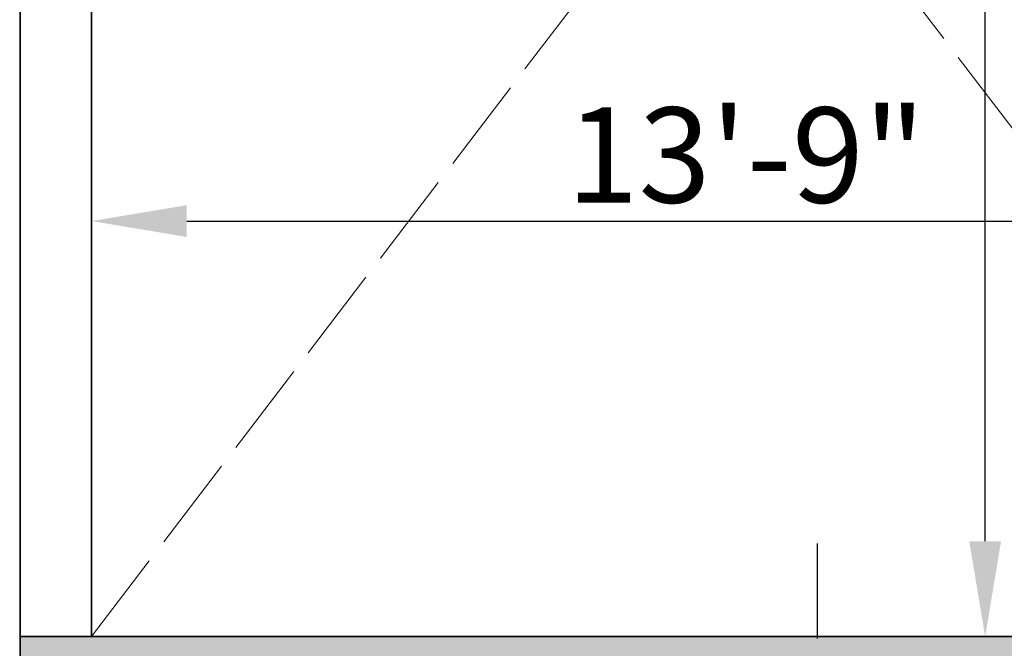
# Model space of a CAD drawing. Units: inches. Extents: x 2083 to 3317, y 1141 to 2115.
# Tile 248 of 256: x 2944 to 3068, y 1485 to 1564. Entities that reach past the tile are written whole.
import ezdxf

# ---------------------------------------------------------------- set-up
doc = ezdxf.new("R2010")
doc.units = ezdxf.units.IN
doc.linetypes.add('ACAD_ISO02W100', pattern=[15, 12, -3])
for name, color, linetype, lineweight in [('A-ANNO-DIMS', 2, 'Continuous', 18), ('A-FLOR-OPEN', 8, 'ACAD_ISO02W100', 13), ('A-WALL', 7, 'Continuous', 35)]:
    doc.layers.add(name, color=color, linetype=linetype, lineweight=lineweight)
doc.layers.add('A-WALL-PATT', color=251, linetype='Continuous', lineweight=13, true_color=0x636466)
doc.styles.get("Standard").update_dxf_attribs({"font": 'arial.ttf'})
doc.dimstyles.new('ISO-25', dxfattribs={"dimtxt": 12, "dimasz": 12, "dimexe": 1.25, "dimexo": 0.625, "dimtad": 1, "dimlunit": 3, "dimtxsty": 'Standard', "dimcen": 2.5, "dimadec": 0, "dimazin": 0, "dimtfac": 1, "dimtmove": 0, "dimatfit": 3, "dimfxl": 1, "dimarcsym": 0})

# ---------------------------------------------------------------- blocks, each defined once
blk = doc.blocks.new('*D18')
at = {"layer": 'A-ANNO-DIMS', "color": 0, "lineweight": -2, "transparency": 16777216}
for p, q in [((3018.48, 1456.16), (3018.48, 1452.14)), ((3041.07, 1456.16), (3041.07, 1452.14)), ((3006.48, 1453.39), (2828.36, 1453.39)), ((3041.07, 1453.39), (3018.48, 1453.39)), ((3053.07, 1453.39), (3065.07, 1453.39))]:
    blk.add_line(p, q, dxfattribs=at)
at = {"layer": 'A-ANNO-DIMS', "color": 0, "transparency": 16777216}
for points in [[(3006.48, 1455.39), (3006.48, 1451.39), (3018.48, 1453.39)], [(3053.07, 1455.39), (3053.07, 1451.39), (3041.07, 1453.39)]]:
    blk.add_solid(points, dxfattribs=at)
at = {"layer": 'Defpoints', "color": 0, "transparency": 16777216}
for p in [(3018.48, 1456.78), (3041.07, 1456.78), (3018.48, 1453.39)]:
    blk.add_point(p, dxfattribs=at)
at = {"layer": 'A-ANNO-DIMS', "color": 0, "transparency": 16777216, "insert": (2911.42, 1460.22), "char_height": 12, "attachment_point": 5}
blk.add_mtext('BASIN 1\'-10 1/2" TYP.', dxfattribs=at)
blk = doc.blocks.new('*D19')
at = {"layer": 'A-ANNO-DIMS', "color": 0, "lineweight": -2, "transparency": 16777216}
for p, q in [((3044.46, 1486.5), (3044.46, 1498.5)), ((3041.69, 1474.5), (3045.71, 1474.5)), ((3044.46, 1474.5), (3044.46, 1456.78)), ((3041.69, 1456.78), (3045.71, 1456.78)), ((3044.46, 1444.78), (3044.46, 1331.55))]:
    blk.add_line(p, q, dxfattribs=at)
at = {"layer": 'A-ANNO-DIMS', "color": 0, "transparency": 16777216}
for points in [[(3042.46, 1486.5), (3046.46, 1486.5), (3044.46, 1474.5)], [(3042.46, 1444.78), (3046.46, 1444.78), (3044.46, 1456.78)]]:
    blk.add_solid(points, dxfattribs=at)
at = {"layer": 'Defpoints', "color": 0, "transparency": 16777216}
for p in [(3041.07, 1474.5), (3041.07, 1456.78), (3044.46, 1456.78)]:
    blk.add_point(p, dxfattribs=at)
at = {"layer": 'A-ANNO-DIMS', "color": 0, "transparency": 16777216, "insert": (3037.63, 1382.17), "char_height": 12, "attachment_point": 5, "rotation": 90}
blk.add_mtext('1\'-5 1/2" TYP.', dxfattribs=at)
blk = doc.blocks.new('*D46')
at = {"layer": 'A-ANNO-DIMS', "color": 0, "lineweight": -2, "transparency": 16777216}
for p, q in [((2952.96, 1487.39), (2952.96, 1540.36)), ((3117.96, 1487.39), (3117.96, 1540.36)), ((2964.96, 1539.11), (3105.96, 1539.11))]:
    blk.add_line(p, q, dxfattribs=at)
at = {"layer": 'A-ANNO-DIMS', "color": 0, "transparency": 16777216}
for points in [[(2964.96, 1541.11), (2964.96, 1537.11), (2952.96, 1539.11)], [(3105.96, 1541.11), (3105.96, 1537.11), (3117.96, 1539.11)]]:
    blk.add_solid(points, dxfattribs=at)
at = {"layer": 'Defpoints', "color": 0, "transparency": 16777216}
for p in [(3117.96, 1539.11), (2952.96, 1486.76), (3117.96, 1486.76)]:
    blk.add_point(p, dxfattribs=at)
at = {"layer": 'A-ANNO-DIMS', "color": 0, "transparency": 16777216, "insert": (3035.46, 1545.87), "char_height": 12, "attachment_point": 5}
blk.add_mtext('13\'-9"', dxfattribs=at)
blk = doc.blocks.new('*D65')
at = {"layer": 'A-ANNO-DIMS', "color": 0, "lineweight": -2, "transparency": 16777216}
for p, q in [((3117.33, 1702.76), (3064.36, 1702.76)), ((3065.61, 1498.76), (3065.61, 1690.76)), ((3117.33, 1486.76), (3064.36, 1486.76))]:
    blk.add_line(p, q, dxfattribs=at)
at = {"layer": 'A-ANNO-DIMS', "color": 0, "transparency": 16777216}
for points in [[(3063.61, 1690.76), (3067.61, 1690.76), (3065.61, 1702.76)], [(3063.61, 1498.76), (3067.61, 1498.76), (3065.61, 1486.76)]]:
    blk.add_solid(points, dxfattribs=at)
at = {"layer": 'Defpoints', "color": 0, "transparency": 16777216}
for p in [(3065.61, 1702.76), (3117.96, 1702.76), (3117.96, 1486.76)]:
    blk.add_point(p, dxfattribs=at)
at = {"layer": 'A-ANNO-DIMS', "color": 0, "transparency": 16777216, "insert": (3058.86, 1594.76), "char_height": 12, "attachment_point": 5, "rotation": 90}
blk.add_mtext('18\'-0"', dxfattribs=at)

msp = doc.modelspace()

# ---------------------------------------------------------------- hatches: boundary and pattern name
at = {"layer": 'A-WALL-PATT'}
h = msp.add_hatch(color=256, dxfattribs=at)
h.dxf.hatch_style = 1
h.paths.add_polyline_path([(3126.96, 2020.761), (2748.96, 2020.761), (2604.96, 2020.761), (2226.96, 2020.761), (2226.96, 1702.761), (2466.96, 1702.761), (2466.96, 1582.761), (2418.96, 1582.761), (2418.96, 1477.761), (2226.96, 1477.761), (2226.96, 1263.261), (2544.96, 1263.261), (2544.96, 1411.761), (2604.96, 1411.761), (2685.96, 1411.761), (2685.96, 1420.761), (2604.96, 1420.761), (2604.96, 1573.761), (2604.96, 1702.761), (2604.96, 2011.761), (2748.96, 2011.761), (2748.96, 1702.761), (2862.96, 1702.761), (2862.96, 1621.761), (2871.96, 1621.761), (2871.96, 1702.761), (2883.96, 1702.761), (2883.96, 1706.939, -0.0264593), (2883.96, 1711.761), (2757.96, 1711.761), (2757.96, 1807.761), (2787.96, 1807.761), (2787.96, 1812.261), (2757.96, 1812.261), (2757.96, 2011.761), (2877.96, 2011.761), (2877.96, 1812.261), (2847.96, 1812.261), (2847.96, 1807.761), (2889.836, 1807.761), (2889.836, 1812.261), (2882.46, 1812.261), (2882.46, 2011.761), (3117.96, 2011.761), (3117.96, 1812.261), (2937.836, 1812.261), (2937.836, 1807.761), (2995.71, 1807.761), (2995.71, 1796.118), (3000.21, 1796.118), (3000.21, 1807.761), (3117.96, 1807.761), (3117.96, 1711.761), (3000.21, 1711.761), (3000.21, 1760.118), (2998.573, 1760.118, -0.020711), (2995.71, 1760.118), (2995.71, 1711.761), (2931.96, 1711.761), (2931.96, 1702.761), (3126.96, 1702.761)])
h.paths.add_polyline_path([(2471.46, 2011.761), (2471.46, 1810.011), (2462.717, 1810.011), (2462.717, 1805.511), (2505.96, 1805.511), (2505.96, 1810.011), (2475.96, 1810.011), (2475.96, 2011.761), (2595.96, 2011.761), (2595.96, 1810.011), (2565.96, 1810.011), (2565.96, 1805.511), (2595.96, 1805.511), (2595.96, 1711.761), (2235.96, 1711.761), (2235.96, 1805.511), (2353.71, 1805.511), (2353.71, 1796.054), (2358.21, 1796.054), (2358.21, 1805.511), (2414.717, 1805.511), (2414.717, 1810.011), (2235.96, 1810.011), (2235.96, 2011.761)], flags=16)
h.paths.add_polyline_path([(2270.205, 1994.61), (2270.205, 1970.61), (2246.205, 1970.61), (2246.205, 1994.61)], flags=0)
edge = h.paths.add_edge_path(flags=0)
edge.add_ellipse((2332.027, 1899.798), major_axis=(-3.043, 3.043), ratio=0.1682525, start_angle=-161.33217, end_angle=-156.30711, ccw=False)
edge.add_ellipse((2333.082, 1898.744), major_axis=(-1.055, 1.055), ratio=0.4535321, start_angle=-123.37102, end_angle=-94.15911)
edge = h.paths.add_edge_path(flags=0)
edge.add_ellipse((2332.027, 1968.876), major_axis=(3.043, 3.043), ratio=0.1682525, start_angle=18.66783, end_angle=23.69289)
edge.add_spline(control_points=[(2332.926, 1970.691), (2332.227, 1970.336), (2330.894, 1969.659), (2328.413, 1970.932), (2327.204, 1967.749), (2324.71, 1969.956), (2322.533, 1967.012), (2320.013, 1971.296), (2317.68, 1968.158), (2316.041, 1967.102), (2315.427, 1966.81)], knot_values=[0, 0, 0, 0, 2.2670587, 4.3245589, 6.6855835, 8.8786411, 11.121502, 14.300359, 17.7552837, 19.732645, 19.732645, 19.732645, 19.732645], degree=3, periodic=0)
edge.add_ellipse((2332.027, 1968.876), major_axis=(3.043, 3.043), ratio=0.1682525, start_angle=18.66783, end_angle=23.69289, ccw=False)
edge.add_ellipse((2333.082, 1969.931), major_axis=(1.055, 1.055), ratio=0.4535321, start_angle=56.62898, end_angle=85.84089, ccw=False)
edge = h.paths.add_edge_path(flags=0)
edge.add_spline(control_points=[(2296.428, 1967.988), (2293.628, 1965.336), (2287.704, 1959.727), (2299.744, 1949.996), (2294.533, 1935.669), (2290.573, 1920.604), (2293.394, 1909.974), (2296.185, 1904.967)], knot_values=[0.0991853, 0.0991853, 0.0991853, 0.0991853, 0.3453009, 0.6198217, 0.9826526, 1.3860932, 1.8105546, 1.8105546, 1.8105546, 1.8105546], degree=3, periodic=0)
edge.add_spline(control_points=[(2296.185, 1904.967), (2297.384, 1902.619), (2298.001, 1901.949), (2298.553, 1901.468)], knot_values=[0.0062457, 0.0062457, 0.0062457, 0.0062457, 0.0554759, 0.0554759, 0.0554759, 0.0554759], degree=3, periodic=0)
edge.add_spline(control_points=[(2298.553, 1901.468), (2297.259, 1900.923), (2295.225, 1900.232), (2293.06, 1900.614), (2292.101, 1900.788), (2292.09, 1900.791)], knot_values=[0.3128349, 0.3128349, 0.3128349, 0.3128349, 0.4017797, 0.4749867, 0.4759027, 0.4759027, 0.4759027, 0.4759027], degree=3, periodic=0)
edge.add_arc((2292.794, 1904.664), 3.937, 215.4209, 259.69818, ccw=False)
edge.add_spline(control_points=[(2289.585, 1902.382), (2289.477, 1902.535), (2289.368, 1902.688), (2289.261, 1902.841)], knot_values=[0.1028719, 0.1028719, 0.1028719, 0.1028719, 0.1168958, 0.1168958, 0.1168958, 0.1168958], degree=3, periodic=0)
edge.add_spline(control_points=[(2289.261, 1902.841), (2288.687, 1902.55), (2287.64, 1902.02), (2285.881, 1901.874), (2283.853, 1901.504), (2281.72, 1899.711), (2278.467, 1899.493), (2276.157, 1901.883), (2272.259, 1899.804), (2267.778, 1901.843), (2262.244, 1900.184), (2257.415, 1901.782), (2254.318, 1900.726), (2253.178, 1900.337)], knot_values=[0, 0, 0, 0, 1.9079767, 3.4771759, 5.261074, 7.9728515, 11.6802485, 13.7179214, 16.9395917, 22.789562, 27.5025027, 33.5952153, 37.1456181, 37.1456181, 37.1456181, 37.1456181], degree=3, periodic=0)
edge.add_line((2253.178, 1900.337), (2250.244, 1902.841))
edge.add_line((2250.244, 1902.841), (2250.244, 1965.833))
edge.add_line((2250.244, 1965.833), (2253.178, 1968.337))
edge.add_spline(control_points=[(2253.178, 1968.337), (2254.318, 1967.948), (2257.415, 1966.892), (2262.244, 1968.49), (2267.778, 1966.831), (2271.527, 1968.537), (2273.876, 1967.828), (2274.207, 1967.728)], knot_values=[0, 0, 0, 0, 0.0901802, 0.2449351, 0.3646438, 0.5132331, 0.5378548, 0.5378548, 0.5378548, 0.5378548], degree=3, periodic=0)
edge.add_arc((2274.353, 1963.793), 3.937, 72.05113, 92.12795, ccw=False)
edge.add_arc((2281.297, 1985.23), 18.596, 252.05113, 288.56572)
edge.add_arc((2292.317, 1956.029), 12.646, 71.02679, 113.77822, ccw=False)
edge = h.paths.add_edge_path(flags=0)
edge.add_spline(control_points=[(2274.899, 1951.856), (2275.066, 1951.617), (2275.233, 1951.377), (2275.398, 1951.136)], knot_values=[1.4099157, 1.4099157, 1.4099157, 1.4099157, 1.4315903, 1.4315903, 1.4315903, 1.4315903], degree=3, periodic=0)
edge.add_spline(control_points=[(2275.398, 1951.136), (2275.792, 1950.562), (2276.179, 1949.984), (2276.546, 1949.397)], knot_values=[1.3582378, 1.3582378, 1.3582378, 1.3582378, 1.4099157, 1.4099157, 1.4099157, 1.4099157], degree=3, periodic=0)
edge.add_line((2276.546, 1949.397), (2277.437, 1947.862))
edge.add_spline(control_points=[(2277.437, 1947.862), (2276.304, 1945.673), (2274.64, 1942.427), (2274.632, 1938.094), (2272.799, 1930.852), (2274.356, 1943.897), (2275.948, 1947.923), (2276.546, 1949.397)], knot_values=[0.0056315, 0.0056315, 0.0056315, 0.0056315, 0.1860139, 0.2660015, 0.3570872, 0.5963902, 0.7397317, 0.7397317, 0.7397317, 0.7397317], degree=3, periodic=0)
edge.add_spline(control_points=[(2276.546, 1949.397), (2276.179, 1949.984), (2275.792, 1950.562), (2275.398, 1951.136)], knot_values=[1.3582378, 1.3582378, 1.3582378, 1.3582378, 1.4099157, 1.4099157, 1.4099157, 1.4099157], degree=3, periodic=0)
edge.add_spline(control_points=[(2275.398, 1951.136), (2274.943, 1950.08), (2274.208, 1948.025), (2273.935, 1944.851), (2272.469, 1937.627), (2273.466, 1945.696), (2274.701, 1951.059), (2274.899, 1951.856)], knot_values=[0.1043639, 0.1043639, 0.1043639, 0.1043639, 0.1896363, 0.2696239, 0.3607096, 0.6000126, 0.6446217, 0.6446217, 0.6446217, 0.6446217], degree=3, periodic=0)
h.paths.add_polyline_path([(2269.168, 1963.128, -0.3575267), (2268.171, 1960.976, -0.0925607), (2268.171, 1939.436, -0.3575267), (2269.168, 1937.285, -0.3575267), (2267.016, 1938.282, -0.1647847), (2254.686, 1938.282, -0.3575267), (2252.534, 1937.285, -0.3575267), (2253.531, 1939.436, -0.0925607), (2253.531, 1960.976, -0.3575267), (2252.534, 1963.128, -0.3575267), (2254.686, 1962.131, -0.1647847), (2267.016, 1962.131, -0.3575267)], flags=0)
h.paths.add_polyline_path([(2248.874, 1967.802), (2248.874, 1957.028), (2249.458, 1957.028), (2249.458, 1911.647), (2248.874, 1911.647), (2248.874, 1900.873), (2246.512, 1900.873, 0.1973271), (2244.15, 1902.457), (2244.15, 1966.218, 0.1973271), (2246.512, 1967.802)], flags=0)
h.paths.add_polyline_path([(2269.168, 1931.389, -0.3575267), (2268.171, 1929.238, -0.0925607), (2268.171, 1907.698, -0.3575267), (2269.168, 1905.547, -0.3575267), (2267.016, 1906.544, -0.1647847), (2254.686, 1906.544, -0.3575267), (2252.534, 1905.547, -0.3575267), (2253.531, 1907.698, -0.0925607), (2253.531, 1929.238, -0.3575267), (2252.534, 1931.389, -0.3575267), (2254.686, 1930.392, -0.1647847), (2267.016, 1930.392, -0.3575267)], flags=0)
edge = h.paths.add_edge_path(flags=0)
edge.add_spline(control_points=[(2276.197, 1906.724), (2276.168, 1909.029), (2276.114, 1913.372), (2270.598, 1924.925), (2273.905, 1919.013), (2275.922, 1916.262), (2275.475, 1912.402), (2277.258, 1910.381), (2276.696, 1908.225), (2276.646, 1906.813), (2276.618, 1906.008)], knot_values=[0, 0, 0, 0, 8.6102597, 16.2212739, 18.8430575, 23.8048978, 27.4408283, 29.3561016, 31.2034776, 33.6506866, 33.6506866, 33.6506866, 33.6506866], degree=3, periodic=0)
edge.add_spline(control_points=[(2276.618, 1906.008), (2276.623, 1905.624), (2276.498, 1904.629), (2275.442, 1903.855), (2274.937, 1903.08), (2274.859, 1902.841)], knot_values=[0.1564884, 0.1564884, 0.1564884, 0.1564884, 0.1843975, 0.2313765, 0.2505985, 0.2505985, 0.2505985, 0.2505985], degree=3, periodic=0)
edge.add_line((2274.859, 1902.841), (2276.506, 1902.841))
edge.add_spline(control_points=[(2276.506, 1902.841), (2276.788, 1903.085), (2277.665, 1904.125), (2278.25, 1904.341), (2277.654, 1908.527), (2278.156, 1906.228), (2278.1, 1905.286), (2278.847, 1904.069), (2277.857, 1903.415), (2277.874, 1902.991), (2277.904, 1902.841)], knot_values=[0.0595743, 0.0595743, 0.0595743, 0.0595743, 0.0807529, 0.1037415, 0.1697201, 0.1760361, 0.2071372, 0.2404744, 0.2623409, 0.2736605, 0.2736605, 0.2736605, 0.2736605], degree=3, periodic=0)
edge.add_line((2277.904, 1902.841), (2280.03, 1902.841))
edge.add_spline(control_points=[(2280.03, 1902.841), (2279.888, 1903.088), (2279.499, 1903.982), (2280.152, 1905.939), (2278.104, 1909.658), (2279.762, 1907.185), (2280.328, 1904.875), (2280.485, 1903.49), (2281.463, 1903.249), (2281.758, 1902.936), (2281.834, 1902.841)], knot_values=[0.013856, 0.013856, 0.013856, 0.013856, 0.0348738, 0.0888667, 0.1078792, 0.1267378, 0.158714, 0.1937575, 0.2174868, 0.2267221, 0.2267221, 0.2267221, 0.2267221], degree=3, periodic=0)
edge.add_spline(control_points=[(2281.834, 1902.841), (2281.788, 1902.827), (2281.647, 1902.783), (2281.396, 1902.859), (2281.088, 1902.985), (2280.721, 1903.061), (2280.333, 1903.026), (2280.125, 1902.899), (2280.03, 1902.841)], knot_values=[0, 0, 0, 0, 0.1441304, 0.435517, 0.7492759, 1.1530457, 1.5483707, 1.878348, 1.878348, 1.878348, 1.878348], degree=3, periodic=0)
edge.add_line((2280.03, 1902.841), (2277.904, 1902.841))
edge.add_spline(control_points=[(2277.904, 1902.841), (2277.893, 1902.796), (2277.865, 1902.68), (2277.607, 1902.687), (2277.274, 1902.801), (2276.838, 1902.62), (2276.584, 1902.789), (2276.506, 1902.841)], knot_values=[0, 0, 0, 0, 0.1271885, 0.3261988, 0.6280094, 1.2435704, 1.5153306, 1.5153306, 1.5153306, 1.5153306], degree=3, periodic=0)
edge.add_line((2276.506, 1902.841), (2274.859, 1902.841))
edge.add_spline(control_points=[(2274.859, 1902.841), (2274.814, 1902.899), (2274.725, 1903.013), (2274.493, 1903.119), (2274.244, 1902.961), (2273.937, 1903.185), (2273.614, 1902.983), (2273.408, 1902.883), (2273.322, 1902.841)], knot_values=[0, 0, 0, 0, 0.2184302, 0.4369566, 0.6879766, 0.9903786, 1.3983955, 1.6918498, 1.6918498, 1.6918498, 1.6918498], degree=3, periodic=0)
edge.add_spline(control_points=[(2273.322, 1902.841), (2273.617, 1903.446), (2274.274, 1904.538), (2276.027, 1904.574), (2276.207, 1906.584), (2276.197, 1906.724)], knot_values=[0.0122268, 0.0122268, 0.0122268, 0.0122268, 0.0594721, 0.1062177, 0.134458, 0.134458, 0.134458, 0.134458], degree=3, periodic=0)
h.paths.add_polyline_path([(2270.776, 1897.79), (2270.776, 1873.79), (2246.776, 1873.79), (2246.776, 1897.79)], flags=0)
h.paths.add_polyline_path([(2353.71, 1760.005), (2353.71, 1760.054), (2358.21, 1760.054, -0.033729)], flags=0)
h.paths.add_polyline_path([(2321.819, 1737.529), (2341.995, 1737.529, -0.4142136), (2343.203, 1736.321), (2343.203, 1721.021, -0.4142136), (2341.995, 1719.813), (2321.819, 1719.813, -0.4142136), (2320.611, 1721.021), (2320.611, 1736.321, -0.4142136)], flags=0)
h.paths.add_polyline_path([(2324.235, 1736.321), (2339.579, 1736.321, -0.4142136), (2341.995, 1733.905), (2341.995, 1725.45, -0.4142136), (2339.579, 1723.034), (2333.681, 1723.034), (2333.845, 1722.045, -0.8706461), (2335.425, 1721.826, -0.767327), (2333.923, 1721.423), (2331.291, 1721.423, -0.767327), (2329.788, 1721.826, -0.8706461), (2331.368, 1722.045), (2331.533, 1723.034), (2324.235, 1723.034, -0.4142136), (2321.819, 1725.45), (2321.819, 1733.905, -0.4142136)], flags=0)
h.paths.add_polyline_path([(2570.484, 1928.615), (2589.684, 1928.615), (2590.169, 1928.615), (2590.169, 1904.993), (2570.484, 1904.993)], flags=0)
h.paths.add_polyline_path([(2574.447, 1927.264, -1), (2572.829, 1927.264, -1)], flags=0)
h.paths.add_polyline_path([(2573.09, 1926.941), (2573.925, 1927.776), (2574.148, 1927.553), (2573.313, 1926.718)], flags=0)
h.paths.add_polyline_path([(2578.779, 1919.73, -1), (2571.592, 1919.73, -1)], flags=0)
h.paths.add_polyline_path([(2578.385, 1919.73, -1), (2571.985, 1919.73, -1)], flags=0)
h.paths.add_polyline_path([(2331.596, 1729.476, -1), (2333.618, 1729.476, -1)], flags=0)
h.paths.add_polyline_path([(2578.034, 1927.264, -1), (2576.416, 1927.264, -1)], flags=0)
h.paths.add_polyline_path([(2576.689, 1927.531), (2576.912, 1927.754), (2577.747, 1926.919), (2577.524, 1926.696)], flags=0)
h.paths.add_polyline_path([(2578.139, 1909.86, -1), (2572.232, 1909.86, -1)], flags=0)
h.paths.add_polyline_path([(2577.745, 1909.86, -1), (2572.625, 1909.86, -1)], flags=0)
h.paths.add_polyline_path([(2583.798, 1927.264, -1), (2582.179, 1927.264, -1)], flags=0)
h.paths.add_polyline_path([(2582.719, 1927.754), (2583.554, 1926.919), (2583.331, 1926.696), (2582.496, 1927.531)], flags=0)
h.paths.add_polyline_path([(2582.496, 1927.531), (2582.719, 1927.754), (2583.554, 1926.919), (2583.331, 1926.696)], flags=0)
h.paths.add_polyline_path([(2587.739, 1920.53, -1), (2581.832, 1920.53, -1)], flags=0)
h.paths.add_polyline_path([(2587.345, 1920.53, -1), (2582.225, 1920.53, -1)], flags=0)
h.paths.add_polyline_path([(2587.385, 1927.264, -1), (2585.766, 1927.264, -1)], flags=0)
h.paths.add_polyline_path([(2586.082, 1926.98), (2586.917, 1927.815), (2587.14, 1927.593), (2586.305, 1926.758)], flags=0)
h.paths.add_polyline_path([(2588.379, 1910.66, -1), (2581.192, 1910.66, -1)], flags=0)
h.paths.add_polyline_path([(2587.985, 1910.66, -1), (2581.585, 1910.66, -1)], flags=0)
h.paths.add_polyline_path([(2417.168, 1729.478), (2437.344, 1729.478, -0.4142136), (2438.552, 1728.27), (2438.552, 1712.969, -0.4142136), (2437.344, 1711.761), (2417.168, 1711.761, -0.4142136), (2415.96, 1712.969), (2415.96, 1728.27, -0.4142136)], flags=0)
h.paths.add_polyline_path([(2419.584, 1728.27), (2434.928, 1728.27, -0.4142136), (2437.344, 1725.854), (2437.344, 1717.398, -0.4142136), (2434.928, 1714.983), (2429.029, 1714.983), (2429.194, 1713.994, -0.8706461), (2430.774, 1713.775, -0.767327), (2429.271, 1713.372), (2426.64, 1713.372, -0.767327), (2425.137, 1713.775, -0.8706461), (2426.717, 1713.994), (2426.882, 1714.983), (2419.584, 1714.983, -0.4142136), (2417.168, 1717.398), (2417.168, 1725.854, -0.4142136)], flags=0)
h.paths.add_polyline_path([(2419.584, 1728.27), (2434.928, 1728.27, -0.4142136), (2437.344, 1725.854), (2437.344, 1717.398, -0.4142136), (2434.928, 1714.983), (2429.029, 1714.983), (2428.358, 1719.009), (2427.553, 1719.009), (2426.882, 1714.983), (2419.584, 1714.983, -0.4142136), (2417.168, 1717.398), (2417.168, 1725.854, -0.4142136)], flags=0)
h.paths.add_polyline_path([(2426.944, 1721.425, -1), (2428.967, 1721.425, -1)], flags=0)
h.paths.add_polyline_path([(2475.96, 1702.761), (2595.96, 1702.761), (2595.96, 1582.761), (2475.96, 1582.761)], flags=16)
h.paths.add_polyline_path([(2427.96, 1573.761), (2595.96, 1573.761), (2595.96, 1468.761), (2595.96, 1420.761), (2384.46, 1420.761), (2384.46, 1468.761), (2427.96, 1468.761)], flags=16)
h.paths.add_polyline_path([(2379.96, 1468.761), (2379.96, 1420.761), (2235.96, 1420.761), (2235.96, 1468.761)], flags=16)
h.paths.add_polyline_path([(2317.816, 1466.696), (2337.992, 1466.696, -0.4142136), (2339.2, 1465.488), (2339.2, 1450.187, -0.4142136), (2337.992, 1448.979), (2317.816, 1448.979, -0.4142136), (2316.608, 1450.187), (2316.608, 1465.488, -0.4142136)], flags=0)
h.paths.add_polyline_path([(2320.232, 1465.488), (2335.576, 1465.488, -0.4142136), (2337.992, 1463.072), (2337.992, 1454.616, -0.4142136), (2335.576, 1452.2), (2329.677, 1452.2), (2329.842, 1451.212, -0.8706461), (2331.422, 1450.992, -0.767327), (2329.92, 1450.59), (2327.288, 1450.59, -0.767327), (2325.785, 1450.992, -0.8706461), (2327.365, 1451.212), (2327.53, 1452.2), (2320.232, 1452.2, -0.4142136), (2317.816, 1454.616), (2317.816, 1463.072, -0.4142136)], flags=0)
h.paths.add_polyline_path([(2320.232, 1465.488), (2335.576, 1465.488, -0.4142136), (2337.992, 1463.072), (2337.992, 1454.616, -0.4142136), (2335.576, 1452.2), (2329.677, 1452.2), (2329.006, 1456.227), (2328.201, 1456.227), (2327.53, 1452.2), (2320.232, 1452.2, -0.4142136), (2317.816, 1454.616), (2317.816, 1463.072, -0.4142136)], flags=0)
h.paths.add_polyline_path([(2327.593, 1458.643, -1), (2329.615, 1458.643, -1)], flags=0)
h.paths.add_polyline_path([(2244.412, 1433.34), (2241.921, 1433.34, -0.4142136), (2240.018, 1435.244), (2240.018, 1440.953, -0.4142105), (2241.921, 1442.856), (2244.412, 1442.856, -1.9764724)], flags=0)
h.paths.add_polyline_path([(2245.357, 1434.398, -0.4142136), (2245.357, 1441.799, -2.1440985)], flags=0)
h.paths.add_polyline_path([(2535.96, 1416.261), (2535.96, 1272.261), (2235.96, 1272.261), (2235.96, 1416.261)], flags=16)
h.paths.add_polyline_path([(2260.12, 1384.293), (2260.12, 1362.039), (2237.865, 1362.039), (2237.865, 1384.293)], flags=0)
edge = h.paths.add_edge_path(flags=0)
edge.add_line((2318.252, 1362.093), (2318.146, 1362.001))
edge.add_ellipse((2317.445, 1360.431), major_axis=(2.822, 2.822), ratio=0.1682525, start_angle=18.66783, end_angle=20.94813, ccw=False)
edge.add_ellipse((2318.423, 1361.409), major_axis=(0.978, 0.978), ratio=0.4535321, start_angle=56.62898, end_angle=70.2262, ccw=False)
edge = h.paths.add_edge_path(flags=0)
edge.add_line((2319.107, 1295.571), (2319.015, 1295.677))
edge.add_ellipse((2317.445, 1296.378), major_axis=(-2.822, 2.822), ratio=0.1682525, start_angle=-161.33217, end_angle=-159.05187, ccw=False)
edge.add_ellipse((2318.423, 1295.4), major_axis=(-0.978, 0.978), ratio=0.4535321, start_angle=-123.37102, end_angle=-109.7738)
edge = h.paths.add_edge_path(flags=0)
edge.add_spline(control_points=[(2284.21, 1301.17), (2284.581, 1300.445), (2284.891, 1299.892), (2285.16, 1299.461)], knot_values=[0.0390658, 0.0390658, 0.0390658, 0.0390658, 0.0554759, 0.0554759, 0.0554759, 0.0554759], degree=3, periodic=0)
edge.add_line((2285.16, 1299.461), (2284.21, 1301.17))
edge = h.paths.add_edge_path(flags=0)
edge.add_line((2280.412, 1297.298), (2283.37, 1297.036))
edge.add_line((2283.37, 1297.036), (2286.406, 1297.926))
edge.add_spline(control_points=[(2286.406, 1297.926), (2285.305, 1297.463), (2284.345, 1297.129), (2283.37, 1297.036)], knot_values=[0.3943688, 0.3943688, 0.3943688, 0.3943688, 0.4759027, 0.4759027, 0.4759027, 0.4759027], degree=3, periodic=0)
edge.add_spline(control_points=[(2283.37, 1297.036), (2283.281, 1297.028), (2282.316, 1296.957), (2281.313, 1297.134), (2280.423, 1297.296), (2280.412, 1297.298)], knot_values=[0.3128349, 0.3128349, 0.3128349, 0.3128349, 0.3202458, 0.3934528, 0.3943688, 0.3943688, 0.3943688, 0.3943688], degree=3, periodic=0)
edge = h.paths.add_edge_path(flags=0)
edge.add_line((2284.436, 1359.607), (2280.446, 1355.328))
edge.add_line((2280.446, 1355.328), (2279.58, 1351.018))
edge.add_line((2279.58, 1351.018), (2282.413, 1346.58))
edge.add_spline(control_points=[(2282.413, 1346.58), (2283.153, 1345.589), (2284.253, 1344.029), (2284.801, 1342.387), (2284.935, 1341.806)], knot_values=[1.2400982, 1.2400982, 1.2400982, 1.2400982, 1.3328922, 1.3827123, 1.3827123, 1.3827123, 1.3827123], degree=3, periodic=0)
edge.add_spline(control_points=[(2284.935, 1341.806), (2285.319, 1340.141), (2285.233, 1338.409), (2284.91, 1336.654)], knot_values=[1.0974841, 1.0974841, 1.0974841, 1.0974841, 1.2400982, 1.2400982, 1.2400982, 1.2400982], degree=3, periodic=0)
edge.add_spline(control_points=[(2284.91, 1336.654), (2284.587, 1334.899), (2284.027, 1333.12), (2283.463, 1331.361)], knot_values=[0.9548699, 0.9548699, 0.9548699, 0.9548699, 1.0974841, 1.0974841, 1.0974841, 1.0974841], degree=3, periodic=0)
edge.add_line((2283.463, 1331.361), (2281.89, 1326.153))
edge.add_line((2281.89, 1326.153), (2280.756, 1321.056))
edge.add_line((2280.756, 1321.056), (2280.299, 1316.002))
edge.add_line((2280.299, 1316.002), (2280.716, 1310.95))
edge.add_line((2280.716, 1310.95), (2282.028, 1305.972))
edge.add_line((2282.028, 1305.972), (2284.21, 1301.17))
edge.add_spline(control_points=[(2284.21, 1301.17), (2283.341, 1302.73), (2282.612, 1304.336), (2282.028, 1305.972)], knot_values=[0.0991853, 0.0991853, 0.0991853, 0.0991853, 0.2417994, 0.2417994, 0.2417994, 0.2417994], degree=3, periodic=0)
edge.add_spline(control_points=[(2282.028, 1305.972), (2281.444, 1307.608), (2281.005, 1309.273), (2280.716, 1310.95)], knot_values=[0.2417994, 0.2417994, 0.2417994, 0.2417994, 0.3844135, 0.3844135, 0.3844135, 0.3844135], degree=3, periodic=0)
edge.add_spline(control_points=[(2280.716, 1310.95), (2280.433, 1312.588), (2280.289, 1314.277), (2280.299, 1315.962), (2280.299, 1316.002)], knot_values=[0.3844135, 0.3844135, 0.3844135, 0.3844135, 0.5236467, 0.5270276, 0.5270276, 0.5270276, 0.5270276], degree=3, periodic=0)
edge.add_spline(control_points=[(2280.299, 1316.002), (2280.312, 1317.687), (2280.478, 1319.368), (2280.756, 1321.056)], knot_values=[0.5270276, 0.5270276, 0.5270276, 0.5270276, 0.6696417, 0.6696417, 0.6696417, 0.6696417], degree=3, periodic=0)
edge.add_spline(control_points=[(2280.756, 1321.056), (2281.035, 1322.744), (2281.426, 1324.44), (2281.89, 1326.153)], knot_values=[0.6696417, 0.6696417, 0.6696417, 0.6696417, 0.8122558, 0.8122558, 0.8122558, 0.8122558], degree=3, periodic=0)
edge.add_spline(control_points=[(2281.89, 1326.153), (2282.264, 1327.533), (2282.788, 1329.262), (2283.353, 1331.018), (2283.463, 1331.361)], knot_values=[0.8122558, 0.8122558, 0.8122558, 0.8122558, 0.9270873, 0.9548699, 0.9548699, 0.9548699, 0.9548699], degree=3, periodic=0)
edge.add_line((2283.463, 1331.361), (2284.91, 1336.654))
edge.add_line((2284.91, 1336.654), (2284.935, 1341.806))
edge.add_line((2284.935, 1341.806), (2282.413, 1346.58))
edge.add_spline(control_points=[(2282.413, 1346.58), (2281.275, 1348.104), (2280.078, 1349.57), (2279.58, 1351.018)], knot_values=[1.3827123, 1.3827123, 1.3827123, 1.3827123, 1.5253264, 1.5253264, 1.5253264, 1.5253264], degree=3, periodic=0)
edge.add_spline(control_points=[(2279.58, 1351.018), (2279.443, 1351.415), (2279.136, 1352.857), (2279.735, 1354.29), (2280.446, 1355.328)], knot_values=[1.5253264, 1.5253264, 1.5253264, 1.5253264, 1.564439, 1.6679405, 1.6679405, 1.6679405, 1.6679405], degree=3, periodic=0)
edge.add_spline(control_points=[(2280.446, 1355.328), (2281.426, 1356.758), (2282.931, 1358.183), (2284.436, 1359.607)], knot_values=[1.6679405, 1.6679405, 1.6679405, 1.6679405, 1.8105546, 1.8105546, 1.8105546, 1.8105546], degree=3, periodic=0)
edge.add_arc((2280.623, 1348.518), 11.726, 71.02679, 113.77822)
edge.add_arc((2270.405, 1375.595), 17.244, 252.05113, 288.56572, ccw=False)
edge.add_arc((2263.966, 1355.718), 3.651, 72.05113, 92.12795)
edge.add_arc((2263.966, 1355.718), 3.651, 92.12795, 177.98513)
edge.add_spline(control_points=[(2260.318, 1355.846), (2260.26, 1354.221), (2260.551, 1350.187), (2262.999, 1346.766), (2264.473, 1344.649)], knot_values=[1.4315903, 1.4315903, 1.4315903, 1.4315903, 1.5641438, 1.7706953, 1.7706953, 1.7706953, 1.7706953], degree=3, periodic=0)
edge.add_line((2264.473, 1344.649), (2264.936, 1343.983))
edge.add_spline(control_points=[(2263.801, 1340.248), (2263.843, 1340.514), (2264.067, 1341.756), (2264.513, 1343.002), (2264.935, 1343.981)], knot_values=[0.5365702, 0.5365702, 0.5365702, 0.5365702, 0.5593494, 0.6446217, 0.6446217, 0.6446217, 0.6446217], degree=3, periodic=0)
edge.add_spline(control_points=[(2264.935, 1343.981), (2265.118, 1343.715), (2265.299, 1343.448), (2265.477, 1343.179)], knot_values=[1.3840767, 1.3840767, 1.3840767, 1.3840767, 1.4099157, 1.4099157, 1.4099157, 1.4099157], degree=3, periodic=0)
edge.add_spline(control_points=[(2265.477, 1343.179), (2265.655, 1342.911), (2265.829, 1342.641), (2265.999, 1342.369)], knot_values=[1.3582378, 1.3582378, 1.3582378, 1.3582378, 1.3840767, 1.3840767, 1.3840767, 1.3840767], degree=3, periodic=0)
edge.add_line((2265.999, 1342.369), (2266.826, 1340.946))
edge.add_spline(control_points=[(2266.826, 1340.946), (2268.894, 1337.09), (2271.398, 1325.843), (2270.516, 1310.569), (2275.919, 1301.861), (2277.79, 1299.199)], knot_values=[0.1168958, 0.1168958, 0.1168958, 0.1168958, 0.4729873, 1.0509689, 1.3137934, 1.3137934, 1.3137934, 1.3137934], degree=3, periodic=0)
edge.add_spline(control_points=[(2277.79, 1299.199), (2277.839, 1299.128), (2277.889, 1299.057), (2277.94, 1298.987)], knot_values=[0.1098839, 0.1098839, 0.1098839, 0.1098839, 0.1168958, 0.1168958, 0.1168958, 0.1168958], degree=3, periodic=0)
edge.add_line((2277.94, 1298.987), (2277.789, 1299.199))
edge.add_spline(control_points=[(2277.789, 1299.199), (2277.257, 1298.929), (2276.286, 1298.438), (2275.039, 1298.334), (2274.383, 1298.239), (2274.215, 1298.209)], knot_values=[33.1218702, 33.1218702, 33.1218702, 33.1218702, 35.0290557, 36.5982549, 37.1448269, 37.1448269, 37.1448269, 37.1448269], degree=3, periodic=0)
edge.add_line((2274.215, 1298.209), (2273.073, 1297.893))
edge.add_spline(control_points=[(2273.073, 1297.893), (2272.323, 1297.58), (2271.039, 1296.511), (2269.248, 1296.226), (2268.423, 1296.375)], knot_values=[26.5325843, 26.5325843, 26.5325843, 26.5325843, 29.198919, 31.8391012, 31.8391012, 31.8391012, 31.8391012], degree=3, periodic=0)
edge.add_line((2268.423, 1296.375), (2263.879, 1297.458))
edge.add_spline(control_points=[(2263.879, 1297.458), (2263.556, 1297.359), (2261.86, 1296.839), (2260.239, 1297.282), (2258.933, 1297.516)], knot_values=[15.9195506, 15.9195506, 15.9195506, 15.9195506, 16.9395917, 21.2260675, 21.2260675, 21.2260675, 21.2260675], degree=3, periodic=0)
edge.add_line((2258.933, 1297.516), (2254.055, 1297.329))
edge.add_spline(control_points=[(2254.055, 1297.329), (2253.756, 1297.296), (2252.114, 1297.165), (2250.462, 1297.544), (2249.13, 1297.668)], knot_values=[5.3065169, 5.3065169, 5.3065169, 5.3065169, 6.2764352, 10.6130337, 10.6130337, 10.6130337, 10.6130337], degree=3, periodic=0)
edge.add_line((2249.13, 1297.668), (2244.332, 1296.878))
edge.add_line((2244.332, 1296.878), (2241.611, 1299.199))
edge.add_line((2241.611, 1299.199), (2241.611, 1357.609))
edge.add_line((2241.611, 1357.609), (2244.332, 1359.931))
edge.add_line((2244.332, 1359.931), (2252.729, 1359.543))
edge.add_spline(control_points=[(2252.729, 1359.543), (2252.871, 1359.546), (2253.306, 1359.548), (2253.74, 1359.514), (2254.032, 1359.482)], knot_values=[0.233291, 0.233291, 0.233291, 0.233291, 0.2449351, 0.2689274, 0.2689274, 0.2689274, 0.2689274], degree=3, periodic=0)
edge.add_line((2254.032, 1359.482), (2259.587, 1359.416))
edge.add_spline(control_points=[(2259.587, 1359.416), (2260.677, 1359.629), (2262.073, 1359.897), (2263.524, 1359.459), (2263.83, 1359.366)], knot_values=[0.4225164, 0.4225164, 0.4225164, 0.4225164, 0.5132331, 0.5378548, 0.5378548, 0.5378548, 0.5378548], degree=3, periodic=0)
edge.add_arc((2263.966, 1355.718), 3.651, 72.05113, 92.12795, ccw=False)
edge.add_arc((2270.405, 1375.595), 17.244, 252.05113, 288.56572)
edge.add_arc((2280.623, 1348.518), 11.726, 71.02679, 113.77822, ccw=False)
h.paths.add_polyline_path([(2240.341, 1359.435), (2240.341, 1349.444), (2240.882, 1349.444), (2240.882, 1307.365), (2240.341, 1307.365), (2240.341, 1297.374), (2238.15, 1297.374, 0.1973271), (2235.96, 1298.843), (2235.96, 1357.966, 0.1973271), (2238.15, 1359.435)], flags=0)
h.paths.add_polyline_path([(2259.158, 1355.101, -0.3575267), (2258.233, 1353.106, -0.0925607), (2258.233, 1333.133, -0.3575267), (2259.158, 1331.138, -0.3575267), (2257.163, 1332.062, -0.1647847), (2245.729, 1332.062, -0.3575267), (2243.735, 1331.138, -0.3575267), (2244.659, 1333.133, -0.0925607), (2244.659, 1353.106, -0.3575267), (2243.735, 1355.101, -0.3575267), (2245.729, 1354.176, -0.1647847), (2257.163, 1354.176, -0.3575267)], flags=0)
edge = h.paths.add_edge_path(flags=0)
edge.add_line((2265.999, 1342.369), (2266.826, 1340.946))
edge.add_line((2266.826, 1340.946), (2265.308, 1337.814))
edge.add_line((2265.308, 1337.814), (2264.358, 1334.653))
edge.add_line((2264.358, 1334.653), (2264.262, 1333.8))
edge.add_spline(control_points=[(2264.262, 1333.8), (2264.208, 1333.187), (2264.162, 1332.366), (2264.007, 1331.414), (2263.969, 1331.202)], knot_values=[0.4644442, 0.4644442, 0.4644442, 0.4644442, 0.5166905, 0.5316081, 0.5316081, 0.5316081, 0.5316081], degree=3, periodic=0)
edge.add_spline(control_points=[(2263.969, 1331.202), (2263.775, 1330.119), (2263.424, 1328.791), (2263.257, 1328.531), (2263.234, 1328.515)], knot_values=[0.3726816, 0.3726816, 0.3726816, 0.3726816, 0.4488497, 0.4644442, 0.4644442, 0.4644442, 0.4644442], degree=3, periodic=0)
edge.add_spline(control_points=[(2263.234, 1328.515), (2263.096, 1328.42), (2263.131, 1329.301), (2263.275, 1330.616)], knot_values=[0.2809191, 0.2809191, 0.2809191, 0.2809191, 0.3726816, 0.3726816, 0.3726816, 0.3726816], degree=3, periodic=0)
edge.add_spline(control_points=[(2263.275, 1330.616), (2263.419, 1331.93), (2263.672, 1333.677), (2263.97, 1335.315)], knot_values=[0.1891566, 0.1891566, 0.1891566, 0.1891566, 0.2809191, 0.2809191, 0.2809191, 0.2809191], degree=3, periodic=0)
edge.add_spline(control_points=[(2263.97, 1335.315), (2264.1, 1336.032), (2264.419, 1337.622), (2264.755, 1338.864), (2264.947, 1339.491)], knot_values=[0.097394, 0.097394, 0.097394, 0.097394, 0.1375775, 0.1891566, 0.1891566, 0.1891566, 0.1891566], degree=3, periodic=0)
edge.add_spline(control_points=[(2264.947, 1339.491), (2265.29, 1340.606), (2265.644, 1341.494), (2265.999, 1342.369)], knot_values=[0.0056315, 0.0056315, 0.0056315, 0.0056315, 0.097394, 0.097394, 0.097394, 0.097394], degree=3, periodic=0)
h.paths.add_polyline_path([(2259.158, 1325.671, -0.3575267), (2258.233, 1323.676, -0.0925607), (2258.233, 1303.703, -0.3575267), (2259.158, 1301.708, -0.3575267), (2257.163, 1302.633, -0.1647847), (2245.729, 1302.633, -0.3575267), (2243.735, 1301.708, -0.3575267), (2244.659, 1303.703, -0.0925607), (2244.659, 1323.676, -0.3575267), (2243.735, 1325.671, -0.3575267), (2245.729, 1324.747, -0.1647847), (2257.163, 1324.747, -0.3575267)], flags=0)
edge = h.paths.add_edge_path(flags=0)
edge.add_spline(control_points=[(2261.709, 1317.311), (2261.679, 1317.418), (2261.762, 1317.389), (2262.491, 1316.09), (2262.962, 1315.301)], knot_values=[14.9558607, 14.9558607, 14.9558607, 14.9558607, 16.2212739, 18.6948259, 18.6948259, 18.6948259, 18.6948259], degree=3, periodic=0)
edge.add_spline(control_points=[(2262.962, 1315.301), (2262.99, 1315.254), (2263.702, 1314.067), (2264.349, 1313.127), (2264.73, 1312.164)], knot_values=[18.6948259, 18.6948259, 18.6948259, 18.6948259, 18.8430575, 22.433791, 22.433791, 22.433791, 22.433791], degree=3, periodic=0)
edge.add_spline(control_points=[(2264.73, 1312.164), (2264.876, 1311.796), (2265.177, 1310.77), (2265.143, 1309.559), (2265.248, 1308.824)], knot_values=[22.433791, 22.433791, 22.433791, 22.433791, 23.8048978, 26.1727562, 26.1727562, 26.1727562, 26.1727562], degree=3, periodic=0)
edge.add_line((2265.248, 1308.824), (2265.851, 1307.172))
edge.add_spline(control_points=[(2265.851, 1307.172), (2266.065, 1306.822), (2266.384, 1306.332), (2266.424, 1305.781), (2266.42, 1305.611)], knot_values=[28.0625624, 28.0625624, 28.0625624, 28.0625624, 29.3561016, 29.9117214, 29.9117214, 29.9117214, 29.9117214], degree=3, periodic=0)
edge.add_spline(control_points=[(2266.42, 1305.611), (2266.416, 1305.433), (2266.394, 1305.25), (2266.365, 1305.066)], knot_values=[29.9117214, 29.9117214, 29.9117214, 29.9117214, 30.4978371, 30.4978371, 30.4978371, 30.4978371], degree=3, periodic=0)
edge.add_line((2266.365, 1305.066), (2266.066, 1302.136))
edge.add_spline(control_points=[(2266.066, 1302.136), (2266.071, 1301.78), (2265.998, 1301.2), (2265.663, 1300.759), (2265.509, 1300.586)], knot_values=[0.1564884, 0.1564884, 0.1564884, 0.1564884, 0.1843975, 0.2035434, 0.2035434, 0.2035434, 0.2035434], degree=3, periodic=0)
edge.add_line((2265.509, 1300.586), (2264.435, 1299.199))
edge.add_line((2264.435, 1299.199), (2265.962, 1299.199))
edge.add_line((2265.962, 1299.199), (2267.336, 1301.175))
edge.add_line((2267.336, 1301.175), (2267.312, 1301.986))
edge.add_spline(control_points=[(2267.312, 1301.986), (2267.261, 1302.862), (2267.16, 1303.737), (2267.271, 1303.326)], knot_values=[0.1262286, 0.1262286, 0.1262286, 0.1262286, 0.1666174, 0.1666174, 0.1666174, 0.1666174], degree=3, periodic=0)
edge.add_spline(control_points=[(2267.271, 1303.326), (2267.28, 1303.294), (2267.31, 1303.175), (2267.373, 1302.884), (2267.406, 1302.683), (2267.418, 1302.601)], knot_values=[0.1666174, 0.1666174, 0.1666174, 0.1666174, 0.1697201, 0.1760361, 0.1807647, 0.1807647, 0.1807647, 0.1807647], degree=3, periodic=0)
edge.add_spline(control_points=[(2267.744, 1300.988), (2267.688, 1301.151), (2267.481, 1301.657), (2267.484, 1302.145), (2267.418, 1302.601)], knot_values=[0.1807647, 0.1807647, 0.1807647, 0.1807647, 0.1937665, 0.2201389, 0.2201389, 0.2201389, 0.2201389], degree=3, periodic=0)
edge.add_line((2267.418, 1302.601), (2267.744, 1300.988))
edge.add_spline(control_points=[(2267.744, 1300.988), (2267.832, 1300.732), (2267.932, 1300.31), (2267.555, 1299.975), (2267.429, 1299.829)], knot_values=[0.2201389, 0.2201389, 0.2201389, 0.2201389, 0.2404744, 0.2548903, 0.2548903, 0.2548903, 0.2548903], degree=3, periodic=0)
edge.add_line((2267.429, 1299.829), (2267.258, 1299.199))
edge.add_line((2267.258, 1299.199), (2269.23, 1299.199))
edge.add_spline(control_points=[(2269.23, 1299.199), (2269.099, 1299.429), (2268.843, 1300.016), (2269.012, 1300.916), (2268.947, 1301.661)], knot_values=[0.013856, 0.013856, 0.013856, 0.013856, 0.0348738, 0.0670726, 0.0670726, 0.0670726, 0.0670726], degree=3, periodic=0)
edge.add_line((2268.947, 1301.661), (2268.432, 1303.603))
edge.add_spline(control_points=[(2268.432, 1303.603), (2268.176, 1304.192), (2267.596, 1305.251), (2268.041, 1304.623), (2268.251, 1304.282)], knot_values=[0.0901547, 0.0901547, 0.0901547, 0.0901547, 0.1078792, 0.1202891, 0.1202891, 0.1202891, 0.1202891], degree=3, periodic=0)
edge.add_spline(control_points=[(2268.251, 1304.282), (2268.361, 1304.105), (2269.058, 1302.918), (2269.383, 1301.59), (2269.521, 1300.776), (2269.575, 1300.556)], knot_values=[0.1202891, 0.1202891, 0.1202891, 0.1202891, 0.1267378, 0.158714, 0.1735056, 0.1735056, 0.1735056, 0.1735056], degree=3, periodic=0)
edge.add_line((2269.575, 1300.556), (2270.686, 1299.421))
edge.add_spline(control_points=[(2270.686, 1299.421), (2270.767, 1299.357), (2270.838, 1299.281), (2270.903, 1299.199)], knot_values=[0.2181597, 0.2181597, 0.2181597, 0.2181597, 0.2267221, 0.2267221, 0.2267221, 0.2267221], degree=3, periodic=0)
edge.add_line((2270.937, 1299.193), (2270.903, 1299.199))
edge.add_spline(control_points=[(2270.903, 1299.199), (2270.86, 1299.186), (2270.73, 1299.146), (2270.496, 1299.216), (2270.272, 1299.308), (2270.121, 1299.348), (2270.063, 1299.36)], knot_values=[0.939174, 0.939174, 0.939174, 0.939174, 1.0833044, 1.3746911, 1.6884499, 1.878348, 1.878348, 1.878348, 1.878348], degree=3, periodic=0)
edge.add_line((2270.063, 1299.36), (2269.23, 1299.199))
edge.add_line((2269.23, 1299.199), (2267.258, 1299.199))
edge.add_spline(control_points=[(2267.258, 1299.199), (2267.248, 1299.157), (2267.223, 1299.05), (2266.984, 1299.057), (2266.809, 1299.116), (2266.677, 1299.109), (2266.637, 1299.105)], knot_values=[0.7576653, 0.7576653, 0.7576653, 0.7576653, 0.8848538, 1.0838641, 1.3856747, 1.5153306, 1.5153306, 1.5153306, 1.5153306], degree=3, periodic=0)
edge.add_spline(control_points=[(2266.637, 1299.105), (2266.485, 1299.089), (2266.236, 1299.017), (2266.035, 1299.151), (2265.962, 1299.199)], knot_values=[0, 0, 0, 0, 0.4859051, 0.7576653, 0.7576653, 0.7576653, 0.7576653], degree=3, periodic=0)
edge.add_line((2265.962, 1299.199), (2264.435, 1299.199))
edge.add_line((2264.435, 1299.199), (2263.858, 1299.367))
edge.add_spline(control_points=[(2263.858, 1299.367), (2263.819, 1299.371), (2263.78, 1299.386), (2263.74, 1299.402)], knot_values=[0.8459249, 0.8459249, 0.8459249, 0.8459249, 0.9786272, 0.9786272, 0.9786272, 0.9786272], degree=3, periodic=0)
edge.add_line((2263.722, 1299.396), (2263.01, 1299.199))
edge.add_spline(control_points=[(2263.01, 1299.199), (2263.246, 1299.683), (2263.506, 1300.128), (2263.873, 1300.408)], knot_values=[0.0122268, 0.0122268, 0.0122268, 0.0122268, 0.0529705, 0.0529705, 0.0529705, 0.0529705], degree=3, periodic=0)
edge.add_spline(control_points=[(2263.873, 1300.408), (2263.932, 1300.453), (2264.084, 1300.553), (2264.255, 1300.624), (2264.36, 1300.665)], knot_values=[0.0529705, 0.0529705, 0.0529705, 0.0529705, 0.0594721, 0.0690861, 0.0690861, 0.0690861, 0.0690861], degree=3, periodic=0)
edge.add_line((2264.36, 1300.665), (2265.142, 1301.078))
edge.add_line((2265.142, 1301.078), (2265.676, 1302.8))
edge.add_line((2265.676, 1302.8), (2265.541, 1305.704))
edge.add_line((2265.541, 1305.704), (2264.803, 1309.328))
edge.add_line((2264.803, 1309.328), (2263.041, 1314.092))
edge.add_spline(control_points=[(2263.041, 1314.092), (2262.384, 1315.671), (2261.796, 1316.998), (2261.709, 1317.311)], knot_values=[11.2168955, 11.2168955, 11.2168955, 11.2168955, 14.9558607, 14.9558607, 14.9558607, 14.9558607], degree=3, periodic=0)
h.paths.add_polyline_path([(2871.96, 1416.261), (2895.91, 1416.261), (2895.91, 1420.761), (2871.96, 1420.761), (2871.96, 1501.761), (2862.96, 1501.761), (2862.96, 1420.761), (2805.96, 1420.761), (2805.96, 1411.761), (2862.96, 1411.761), (2862.96, 1263.261), (3126.96, 1263.261), (3126.96, 1411.761), (3126.96, 1486.761), (2943.96, 1486.761), (2943.96, 1477.761), (2967.86, 1477.761), (2967.86, 1420.761), (2943.91, 1420.761), (2943.91, 1416.261), (3117.96, 1416.261), (3117.96, 1420.761), (2972.36, 1420.761), (2972.36, 1477.761), (3117.96, 1477.761), (3117.96, 1420.761), (3117.96, 1272.261), (2871.96, 1272.261)], flags=0)
h.paths.add_polyline_path([(2457.126, 1485.943), (2527.603, 1485.943), (2527.603, 1537.636), (2457.126, 1537.636)], flags=8)
h.paths.add_polyline_path([(2481.005, 1609.982), (2590.766, 1609.982), (2590.766, 1682.003), (2481.005, 1682.003)], flags=8)
h.paths.add_polyline_path([(2483.085, 1729.127), (2553.562, 1729.127), (2553.562, 1780.82), (2483.085, 1780.82)], flags=8)
h = msp.add_hatch(color=256, dxfattribs=at)
h.dxf.hatch_style = 1
h.paths.add_polyline_path([(3126.96, 1486.761), (2943.96, 1486.761), (2943.96, 1477.761), (2967.86, 1477.761), (2967.86, 1420.761), (2943.91, 1420.761), (2943.91, 1416.261), (3117.96, 1416.261), (3117.96, 1420.761), (2972.36, 1420.761), (2972.36, 1477.761), (3117.96, 1477.761), (3117.96, 1420.761), (3117.96, 1272.261), (2871.96, 1272.261), (2871.96, 1416.261), (2895.91, 1416.261), (2895.91, 1420.761), (2871.96, 1420.761), (2871.96, 1501.761), (2862.96, 1501.761), (2862.96, 1420.761), (2805.96, 1420.761), (2805.96, 1411.761), (2862.96, 1411.761), (2862.96, 1263.261), (3126.96, 1263.261), (3126.96, 1411.761)])

# ---------------------------------------------------------------- linework, layer by layer
at = {"layer": 'A-FLOR-OPEN'}
for p, q in [((2952.96, 1486.761), (3117.96, 1702.761)), ((2952.96, 1702.761), (3117.96, 1486.761))]:
    msp.add_line(p, q, dxfattribs=at)
at = {"layer": 'A-WALL'}
for p, q in [((2943.96, 1702.761), (2943.96, 1477.761)), ((2952.96, 1702.761), (2952.96, 1486.761)), ((2943.96, 1486.761), (3126.96, 1486.761))]:
    msp.add_line(p, q, dxfattribs=at)

# ---------------------------------------------------------------- dimensions: what is measured, and where the dimension line sits
at = {"layer": 'A-ANNO-DIMS'}
dim = msp.add_linear_dim(base=(3065.61, 1702.761), p1=(3117.96, 1486.761), p2=(3117.96, 1702.761), angle=90, dimstyle='ISO-25', override={"dimdec": 1, "dimlfac": 1, "dimrnd": 0, "dimzin": 1, "dimdsep": 46, "dimlunit": 4, "dimfrac": 2}, dxfattribs=at)
dim.commit()
dim.dimension.update_dxf_attribs({"geometry": '*D65', "text_midpoint": (3058.858, 1594.761)})
dim = msp.add_linear_dim(base=(3117.96, 1539.111), p1=(2952.96, 1486.761), p2=(3117.96, 1486.761), dimstyle='ISO-25', override={"dimdec": 1, "dimlfac": 1, "dimrnd": 0, "dimzin": 1, "dimdsep": 46, "dimlunit": 4, "dimfrac": 2}, dxfattribs=at)
dim.commit()
dim.dimension.update_dxf_attribs({"geometry": '*D46', "text_midpoint": (3035.46, 1545.867)})
for base, p1, p2, angle, text, picture, middle in [((3018.476, 1453.392), (3041.068, 1456.781), (3018.476, 1456.781), 180, 'BASIN <> TYP.', '*D18', (2911.418, 1460.222)), ((3044.457, 1456.781), (3041.068, 1474.497), (3041.068, 1456.781), 270, '<> TYP.', '*D19', (3037.627, 1382.167))]:
    dim = msp.add_linear_dim(base=base, p1=p1, p2=p2, angle=angle, text=text, dimstyle='ISO-25', override={"dimdec": 1, "dimlfac": 1, "dimrnd": 0, "dimzin": 1, "dimdsep": 46, "dimlunit": 4, "dimfrac": 2}, dxfattribs=at)
    dim.commit()
    dim.dimension.update_dxf_attribs({"geometry": picture, "text_midpoint": middle})

doc.saveas('drawing.dxf')
